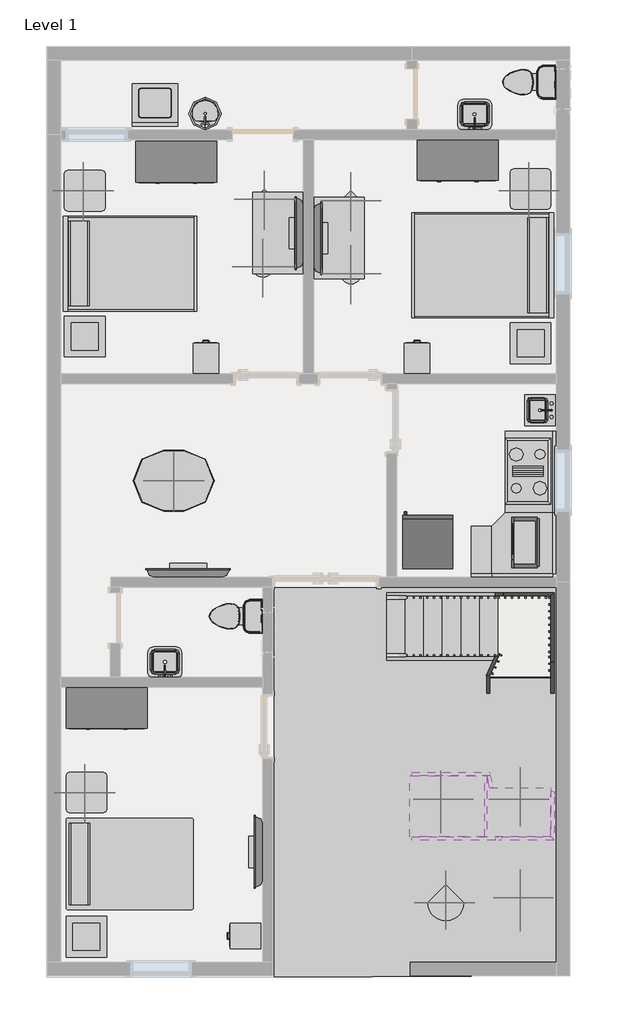
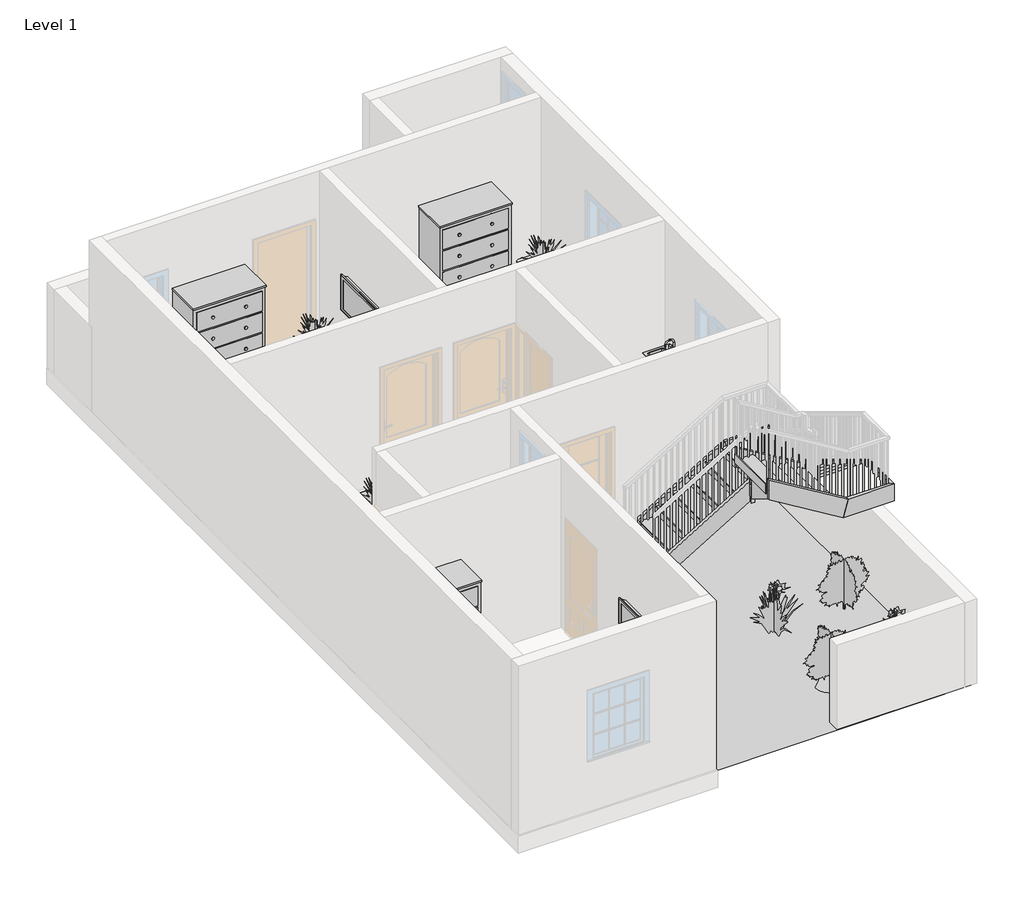
# One storey, part 4 of 4: 23 furniture elements, 12 geographic elements, 12 members, 9 flow terminals, 5 proxies, 3 stair flights, 2 slabs.
"""IFC4 building model written with IfcOpenShell, lengths in millimetres."""

from ifc_helpers import new_model, si_unit, frame, origin, place, context, project, spatial, polyline, outline, extrude, faceted_brep, triangles, transform, mapped, element, save
from components import proxy_bb1e6e30, proxy_8a8d5ab2, proxy_a13a33b2, proxy_718fa39f, flow_terminal_accce45a, flow_terminal_871c2e40, flow_terminal_d49f872f, flow_terminal_62a433f7, toilet_domestic_3d_toilet_domestic_3d_f7549cf7, toilet_domestic_3d_toilet_domestic_3d_183bbd19, furniture_096e7f55, furniture_35c09872, furniture_0253826f, furniture_bb55ed6b, furniture_9fa109b2, furniture_7a3aaa4f, furniture_fdf74506, furniture_b5c51a22, furniture_be1c6672, furniture_31d08a24, furniture_3f969c1c, furniture_25b31cd6, rpc_plant_tropical_55f6ff97, rpc_plant_tropical_agave_1_5_93a2a214, rpc_plant_tropical_jungle_flame_3_9c4808c2, non_monolithic_landing_39c3fcf1, non_monolithic_landing_1f105fa5, stair_flight_290ad292, stair_flight_6c6ed0d7, stair_flight_c4ab4097

model = new_model("IFC4")

# Units and contexts
model_context = context("Model", 3, world=origin())
ifc_project = project(units=[si_unit("LENGTHUNIT", "METRE", prefix="MILLI")], contexts=[model_context])

# Site, building, storey
site = spatial("IfcSite", under=ifc_project)
building = spatial("IfcBuilding", under=site)
storey = spatial("IfcBuildingStorey", under=building, Name="Level 1", Elevation=0.0)

# Proxies
placement = place(None, origin())
element("IfcBuildingElementProxy", 1, Name="Building Element Proxy", at=placement, inside=storey, context=model_context, shape_type="Tessellation", body=[
    triangles([(-10921.0113007, 5381.5366333, 0.0), (-6488.7120758, 5381.5366333, 0.0), (-6488.7120758, -435.0631608, 0.0), (-10921.0113007, -460.4631366, 0.0)], [[1, 4, 3], [3, 2, 1]], closed=False),
])
proxy_shape = proxy_bb1e6e30(model_context)
element("IfcBuildingElementProxy", 2, Name="Cook Top-4 Unit : 36\" x 20\"", ObjectType="Cook Top-4 Unit : 36\" x 20\"", at=placement, inside=storey, context=model_context, shape_type="MappedRepresentation", body=[
    mapped(proxy_shape, transform((-7111.0118598, 7121.4368529, 0.0), x_axis=(0.0, -1.0000000000000004, 0.0), y_axis=(1.0000000000000004, 0.0, 0.0), z_axis=(0.0, 0.0, 1.0))),
])
proxy_2_shape = proxy_8a8d5ab2(model_context)
element("IfcBuildingElementProxy", 3, Name="Microwave : 30\" x 16\" x 18\"", ObjectType="Microwave : 30\" x 16\" x 18\"", at=placement, inside=storey, context=model_context, shape_type="MappedRepresentation", body=[
    mapped(proxy_2_shape, transform((-6796.031354, 6554.9297302, 0.0), x_axis=(0.0, -1.0000000000000004, 0.0), y_axis=(1.0000000000000004, 0.0, 0.0), z_axis=(0.0, 0.0, 1.0))),
])
proxy_3_shape = proxy_a13a33b2(model_context)
element("IfcBuildingElementProxy", 4, Name="Refrigerator : 30\" x 32\" RH", ObjectType="Refrigerator : 30\" x 32\" RH", at=placement, inside=storey, context=model_context, shape_type="MappedRepresentation", body=[
    mapped(proxy_3_shape, transform((-8614.7628883, 6046.6993529, 0.0), x_axis=(-1.0000000000000002, 0.0, 0.0), y_axis=(0.0, -1.0000000000000002, 0.0), z_axis=(0.0, 0.0, 1.0))),
])
proxy_4_shape = proxy_718fa39f(model_context)
element("IfcBuildingElementProxy", 5, Name="Washer : 27\" x 25\" x 35\"", ObjectType="Washer : 27\" x 25\" x 35\"", at=placement, inside=storey, context=model_context, shape_type="MappedRepresentation", body=[
    mapped(proxy_4_shape, transform((-12278.5943913, 12886.9864177, 0.0), x_axis=(-1.0000000000000004, 0.0, 0.0), y_axis=(0.0, -1.0000000000000004, 0.0), z_axis=(0.0, 0.0, 1.0))),
])

# Flow terminals
flow_terminal_shape = flow_terminal_accce45a(model_context)
element("IfcFlowTerminal", 6, ObjectType="Floor Drain - Round : 5\" Strainer - 2\" Drain", at=placement, inside=storey, context=model_context, shape_type="MappedRepresentation", body=[
    mapped(flow_terminal_shape, transform((-12178.3118598, 13077.7368529, 0.0), x_axis=(1.0, 0.0, 0.0), y_axis=(0.0, 1.0, 0.0), z_axis=(0.0, 0.0, 1.0))),
])
element("IfcFlowTerminal", 7, ObjectType="Floor Drain - Round : 5\" Strainer - 2\" Drain", at=placement, inside=storey, context=model_context, shape_type="MappedRepresentation", body=[
    mapped(flow_terminal_shape, transform((-7682.5118598, 13153.9368529, 0.0), x_axis=(1.0, 0.0, 0.0), y_axis=(0.0, 1.0, 0.0), z_axis=(0.0, 0.0, 1.0))),
])
element("IfcFlowTerminal", 8, ObjectType="Floor Drain - Round : 5\" Strainer - 2\" Drain", at=placement, inside=storey, context=model_context, shape_type="MappedRepresentation", body=[
    mapped(flow_terminal_shape, transform((-11441.7118598, 4238.5368529, 0.0), x_axis=(1.0, 0.0, 0.0), y_axis=(0.0, 1.0, 0.0), z_axis=(0.0, 0.0, 1.0))),
])
flow_terminal_2_shape = flow_terminal_871c2e40(model_context)
element("IfcFlowTerminal", 9, ObjectType="Sink Kitchen-Island : 18\" x 18\"", at=placement, inside=storey, context=model_context, shape_type="MappedRepresentation", body=[
    mapped(flow_terminal_2_shape, transform((-6935.5572609, 8051.5260934, 0.0), x_axis=(0.0, -1.0, 0.0), y_axis=(1.0, 0.0, 0.0), z_axis=(0.0, 0.0, 1.0))),
])
flow_terminal_3_shape = flow_terminal_d49f872f(model_context)
element("IfcFlowTerminal", 10, ObjectType="Sink Vanity-Round : 19\" x 19\"", at=placement, inside=storey, context=model_context, shape_type="MappedRepresentation", body=[
    mapped(flow_terminal_3_shape, transform((-11853.0601192, 12566.2547206, 0.0), x_axis=(-1.0000000000000004, 0.0, 0.0), y_axis=(0.0, -1.0000000000000004, 0.0), z_axis=(0.0, 0.0, 1.0))),
])
flow_terminal_4_shape = flow_terminal_62a433f7(model_context)
element("IfcFlowTerminal", 11, ObjectType="Sink Vanity-Square : 20\" x 18\"", at=placement, inside=storey, context=model_context, shape_type="MappedRepresentation", body=[
    mapped(flow_terminal_4_shape, transform((-7895.4226192, 12419.682254, 0.0), x_axis=(-1.0000000000000002, 0.0, 0.0), y_axis=(0.0, -1.0000000000000002, 0.0), z_axis=(0.0, 0.0, 1.0))),
])
element("IfcFlowTerminal", 12, ObjectType="Sink Vanity-Square : 20\" x 18\"", at=placement, inside=storey, context=model_context, shape_type="MappedRepresentation", body=[
    mapped(flow_terminal_4_shape, transform((-12536.3431487, 4215.482254, 0.0), x_axis=(-1.0, 0.0, 0.0), y_axis=(0.0, -1.0, 0.0), z_axis=(0.0, 0.0, 1.0))),
])
toilet_domestic_3d_toilet_domestic_3d_shape = toilet_domestic_3d_toilet_domestic_3d_f7549cf7(model_context)
toilet_domestic_3d_toilet_domestic_3d_2_shape = toilet_domestic_3d_toilet_domestic_3d_183bbd19(model_context)
element("IfcFlowTerminal", 13, ObjectType="Toilet-Domestic-3D : Toilet-Domestic-3D", at=placement, inside=storey, context=model_context, shape_type="MappedRepresentation", body=[
    mapped(toilet_domestic_3d_toilet_domestic_3d_shape, transform((-7186.6078871, 12950.7368529, 0.0), x_axis=(0.0, -1.0000000000000004, 0.0), y_axis=(1.0000000000000004, 0.0, 0.0), z_axis=(0.0, 0.0, 1.0))),
    mapped(toilet_domestic_3d_toilet_domestic_3d_2_shape, transform((-7186.6078871, 12950.7368529, 0.0), x_axis=(0.0, -1.0000000000000004, 0.0), y_axis=(1.0000000000000004, 0.0, 0.0), z_axis=(0.0, 0.0, 1.0))),
])
element("IfcFlowTerminal", 14, ObjectType="Toilet-Domestic-3D : Toilet-Domestic-3D", at=placement, inside=storey, context=model_context, shape_type="MappedRepresentation", body=[
    mapped(toilet_domestic_3d_toilet_domestic_3d_shape, transform((-11580.8078871, 4949.7368529, 0.0), x_axis=(0.0, -1.0000000000000004, 0.0), y_axis=(1.0000000000000004, 0.0, 0.0), z_axis=(0.0, 0.0, 1.0))),
    mapped(toilet_domestic_3d_toilet_domestic_3d_2_shape, transform((-11580.8078871, 4949.7368529, 0.0), x_axis=(0.0, -1.0000000000000004, 0.0), y_axis=(1.0000000000000004, 0.0, 0.0), z_axis=(0.0, 0.0, 1.0))),
])

# Furniture
furniture_shape = furniture_096e7f55(model_context)
element("IfcFurniture", 15, ObjectType="Bed-Shaker : Double 56\" x 78\"", at=placement, inside=storey, context=model_context, shape_type="MappedRepresentation", body=[
    mapped(furniture_shape, transform((-14057.9118598, 10251.9868529, 0.0), x_axis=(0.0, 1.0000000000000002, 0.0), y_axis=(-1.0000000000000002, 0.0, 0.0), z_axis=(0.0, 0.0, 1.0))),
])
furniture_2_shape = furniture_35c09872(model_context)
element("IfcFurniture", 16, ObjectType="Bed-Shaker : Queen 62\" x 83\"", at=placement, inside=storey, context=model_context, shape_type="MappedRepresentation", body=[
    mapped(furniture_2_shape, transform((-6742.7118598, 10188.4868529, 0.0), x_axis=(0.0, -1.0, 0.0), y_axis=(1.0, 0.0, 0.0), z_axis=(0.0, 0.0, 1.0))),
])
furniture_3_shape = furniture_0253826f(model_context)
element("IfcFurniture", 17, ObjectType="Bed-Standard : Double 54\" x 75\"", at=placement, inside=storey, context=model_context, shape_type="MappedRepresentation", body=[
    mapped(furniture_3_shape, transform((-13125.6069417, 969.8483283, 0.0), x_axis=(0.0, 1.0, 0.0), y_axis=(-1.0, 0.0, 0.0), z_axis=(0.0, 0.0, 1.0))),
])
furniture_4_shape = furniture_bb55ed6b(model_context)
element("IfcFurniture", 18, ObjectType="Cabinet-File 2 Drawer : 15\" x 18\"", at=placement, inside=storey, context=model_context, shape_type="MappedRepresentation", body=[
    mapped(furniture_4_shape, transform((-12064.9083068, 8668.4025527, 0.0), x_axis=(-1.0000000000000009, 0.0, 0.0), y_axis=(0.0, -1.0000000000000009, 0.0), z_axis=(0.0, 0.0, 1.0))),
])
element("IfcFurniture", 19, ObjectType="Cabinet-File 2 Drawer : 15\" x 18\"", at=placement, inside=storey, context=model_context, shape_type="MappedRepresentation", body=[
    mapped(furniture_4_shape, transform((-8902.6083068, 8668.4025527, 0.0), x_axis=(-1.0, 0.0, 0.0), y_axis=(0.0, -1.0, 0.0), z_axis=(0.0, 0.0, 1.0))),
])
element("IfcFurniture", 20, ObjectType="Cabinet-File 2 Drawer : 15\" x 18\"", at=placement, inside=storey, context=model_context, shape_type="MappedRepresentation", body=[
    mapped(furniture_4_shape, transform((-11204.3275597, 33.9404058, 0.0), x_axis=(0.0, -0.9999999999999997, 0.0), y_axis=(0.9999999999999997, 0.0, 0.0), z_axis=(0.0, 0.0, 1.0))),
])
furniture_5_shape = furniture_9fa109b2(model_context)
element("IfcFurniture", 21, ObjectType="Dresser : 48\" x 72\" x 24\"", at=placement, inside=storey, context=model_context, shape_type="MappedRepresentation", body=[
    mapped(furniture_5_shape, transform((-12112.3185999, 12120.099807, 0.0), x_axis=(1.0000000000000007, 0.0, 0.0), y_axis=(0.0, 1.0000000000000007, 0.0), z_axis=(0.0, 0.0, 1.0))),
])
element("IfcFurniture", 22, ObjectType="Dresser : 48\" x 72\" x 24\"", at=placement, inside=storey, context=model_context, shape_type="MappedRepresentation", body=[
    mapped(furniture_5_shape, transform((-7895.9185999, 12145.499807, 0.0), x_axis=(1.0, 0.0, 0.0), y_axis=(0.0, 1.0, 0.0), z_axis=(0.0, 0.0, 1.0))),
])
element("IfcFurniture", 23, ObjectType="Dresser : 48\" x 72\" x 24\"", at=placement, inside=storey, context=model_context, shape_type="MappedRepresentation", body=[
    mapped(furniture_5_shape, transform((-13153.7185999, 3941.299807, 0.0), x_axis=(1.0, 0.0, 0.0), y_axis=(0.0, 1.0, 0.0), z_axis=(0.0, 0.0, 1.0))),
])
furniture_6_shape = furniture_7a3aaa4f(model_context)
element("IfcFurniture", 24, ObjectType="TV - Flat Screen : 42\"", at=placement, inside=storey, context=model_context, shape_type="MappedRepresentation", body=[
    mapped(furniture_6_shape, transform((-10535.0504834, 10686.1923387, 1041.4), x_axis=(0.0, -1.0000000000000004, 0.0), y_axis=(1.0000000000000004, 0.0, 0.0), z_axis=(0.0, 0.0, 1.0))),
])
element("IfcFurniture", 25, ObjectType="TV - Flat Screen : 42\"", at=placement, inside=storey, context=model_context, shape_type="MappedRepresentation", body=[
    mapped(furniture_6_shape, transform((-10265.5732361, 10617.881367, 1041.4), x_axis=(0.0, 1.0000000000000002, 0.0), y_axis=(-1.0000000000000002, 0.0, 0.0), z_axis=(0.0, 0.0, 1.0))),
])
element("IfcFurniture", 26, ObjectType="TV - Flat Screen : 42\"", at=placement, inside=storey, context=model_context, shape_type="MappedRepresentation", body=[
    mapped(furniture_6_shape, transform((-11144.6504834, 1415.1923387, 1041.4), x_axis=(0.0, -1.0000000000000004, 0.0), y_axis=(1.0000000000000004, 0.0, 0.0), z_axis=(0.0, 0.0, 1.0))),
])
furniture_7_shape = furniture_fdf74506(model_context)
element("IfcFurniture", 27, ObjectType="TV - Flat Screen : 50\"", at=placement, inside=storey, context=model_context, shape_type="MappedRepresentation", body=[
    mapped(furniture_7_shape, transform((-12207.6563739, 5592.4754765, 1041.4), x_axis=(-1.0000000000000004, 0.0, 0.0), y_axis=(0.0, -1.0000000000000004, 0.0), z_axis=(0.0, 0.0, 1.0))),
])
furniture_8_shape = furniture_b5c51a22(model_context)
element("IfcFurniture", 28, ObjectType="Table-Coffee : 24\" x 24\" x 24\"", at=placement, inside=storey, context=model_context, shape_type="MappedRepresentation", body=[
    mapped(furniture_8_shape, transform((-13771.3776265, 9045.5257751, 0.0), x_axis=(1.0, 0.0, 0.0), y_axis=(0.0, 1.0, 0.0), z_axis=(0.0, 0.0, 1.0))),
])
element("IfcFurniture", 29, ObjectType="Table-Coffee : 24\" x 24\" x 24\"", at=placement, inside=storey, context=model_context, shape_type="MappedRepresentation", body=[
    mapped(furniture_8_shape, transform((-7091.1776265, 8943.9257751, 0.0), x_axis=(1.0, 0.0, 0.0), y_axis=(0.0, 1.0, 0.0), z_axis=(0.0, 0.0, 1.0))),
])
element("IfcFurniture", 30, ObjectType="Table-Coffee : 24\" x 24\" x 24\"", at=placement, inside=storey, context=model_context, shape_type="MappedRepresentation", body=[
    mapped(furniture_8_shape, transform((-13745.9776265, 53.9257751, 0.0), x_axis=(1.0, 0.0, 0.0), y_axis=(0.0, 1.0, 0.0), z_axis=(0.0, 0.0, 1.0))),
])
furniture_9_shape = furniture_be1c6672(model_context)
element("IfcFurniture", 31, ObjectType="Table-Dining Oval : 36\" x 48\"", at=placement, inside=storey, context=model_context, shape_type="MappedRepresentation", body=[
    mapped(furniture_9_shape, transform((-12821.4315319, 6623.6384922, 0.0), x_axis=(-1.0000000000000004, 0.0, 0.0), y_axis=(0.0, -1.0000000000000004, 0.0), z_axis=(0.0, 0.0, 1.0))),
])
furniture_10_shape = furniture_31d08a24(model_context)
element("IfcFurniture", 32, ObjectType="Table-End : 24\" x 24\"", at=placement, inside=storey, context=model_context, shape_type="MappedRepresentation", body=[
    mapped(furniture_10_shape, transform((-14061.6454901, 11172.7368529, 0.0), x_axis=(1.0, 0.0, 0.0), y_axis=(0.0, 1.0, 0.0), z_axis=(0.0, 0.0, 1.0))),
])
element("IfcFurniture", 33, ObjectType="Table-End : 24\" x 24\"", at=placement, inside=storey, context=model_context, shape_type="MappedRepresentation", body=[
    mapped(furniture_10_shape, transform((-7381.4454901, 11198.1368529, 0.0), x_axis=(1.0, 0.0, 0.0), y_axis=(0.0, 1.0, 0.0), z_axis=(0.0, 0.0, 1.0))),
])
element("IfcFurniture", 34, ObjectType="Table-End : 24\" x 24\"", at=placement, inside=storey, context=model_context, shape_type="MappedRepresentation", body=[
    mapped(furniture_10_shape, transform((-14036.2454901, 2155.7368529, 0.0), x_axis=(1.0, 0.0, 0.0), y_axis=(0.0, 1.0, 0.0), z_axis=(0.0, 0.0, 1.0))),
])
furniture_11_shape = furniture_3f969c1c(model_context)
element("IfcFurniture", 35, ObjectType="Table-Rectangular : 72\" x 30\"", at=placement, inside=storey, context=model_context, shape_type="MappedRepresentation", body=[
    mapped(furniture_11_shape, transform((-10857.5118598, 10690.1368529, 0.0), x_axis=(0.0, 1.0000000000000002, 0.0), y_axis=(-1.0000000000000002, 0.0, 0.0), z_axis=(0.0, 0.0, 1.0))),
])
element("IfcFurniture", 36, ObjectType="Table-Rectangular : 72\" x 30\"", at=placement, inside=storey, context=model_context, shape_type="MappedRepresentation", body=[
    mapped(furniture_11_shape, transform((-9943.1118598, 10613.9368529, 0.0), x_axis=(0.0, 1.0000000000000002, 0.0), y_axis=(-1.0000000000000002, 0.0, 0.0), z_axis=(0.0, 0.0, 1.0))),
])
furniture_12_shape = furniture_25b31cd6(model_context)
element("IfcFurniture", 37, ObjectType="Work Station Cubicle : 96\" x 96\"", at=placement, inside=storey, context=model_context, shape_type="MappedRepresentation", body=[
    mapped(furniture_12_shape, transform((-6823.643612, 5038.9138452, 0.0), x_axis=(-1.0000000000000004, 0.0, 0.0), y_axis=(0.0, -1.0000000000000004, 0.0), z_axis=(0.0, 0.0, 1.0))),
])

# Geographic elements
rpc_plant_tropical_shape = rpc_plant_tropical_55f6ff97(model_context)
element("IfcGeographicElement", 38, ObjectType="RPC Plant - Tropical", at=placement, inside=storey, context=model_context, shape_type="MappedRepresentation", body=[
    mapped(rpc_plant_tropical_shape, transform((-8419.1118598, 2206.5368529, 0.0), x_axis=(1.0, 0.0, 0.0), y_axis=(0.0, 1.0, 0.0), z_axis=(0.0, 0.0, 1.0))),
])
element("IfcGeographicElement", 39, ObjectType="RPC Plant - Tropical", at=placement, inside=storey, context=model_context, shape_type="MappedRepresentation", body=[
    mapped(rpc_plant_tropical_shape, transform((-7225.3118598, 733.3368529, 0.0), x_axis=(1.0, 0.0, 0.0), y_axis=(0.0, 1.0, 0.0), z_axis=(0.0, 0.0, 1.0))),
])
rpc_plant_tropical_agave_1_5_shape = rpc_plant_tropical_agave_1_5_93a2a214(model_context)
element("IfcGeographicElement", 40, ObjectType="RPC Plant - Tropical : Agave - 1.5'", at=placement, inside=storey, context=model_context, shape_type="MappedRepresentation", body=[
    mapped(rpc_plant_tropical_agave_1_5_shape, transform((-13778.5118598, 11325.1368529, 609.6), x_axis=(1.0, 0.0, 0.0), y_axis=(0.0, 1.0, 0.0), z_axis=(0.0, 0.0, 1.0))),
])
element("IfcGeographicElement", 41, ObjectType="RPC Plant - Tropical : Agave - 1.5'", at=placement, inside=storey, context=model_context, shape_type="MappedRepresentation", body=[
    mapped(rpc_plant_tropical_agave_1_5_shape, transform((-11060.7118598, 11198.1368529, 660.4), x_axis=(1.0, 0.0, 0.0), y_axis=(0.0, 1.0, 0.0), z_axis=(0.0, 0.0, 1.0))),
])
element("IfcGeographicElement", 42, ObjectType="RPC Plant - Tropical : Agave - 1.5'", at=placement, inside=storey, context=model_context, shape_type="MappedRepresentation", body=[
    mapped(rpc_plant_tropical_agave_1_5_shape, transform((-11086.1118598, 10182.1368529, 660.4), x_axis=(1.0, 0.0, 0.0), y_axis=(0.0, 1.0, 0.0), z_axis=(0.0, 0.0, 1.0))),
])
element("IfcGeographicElement", 43, ObjectType="RPC Plant - Tropical : Agave - 1.5'", at=placement, inside=storey, context=model_context, shape_type="MappedRepresentation", body=[
    mapped(rpc_plant_tropical_agave_1_5_shape, transform((-7098.3118598, 11325.1368529, 609.6), x_axis=(1.0, 0.0, 0.0), y_axis=(0.0, 1.0, 0.0), z_axis=(0.0, 0.0, 1.0))),
])
element("IfcGeographicElement", 44, ObjectType="RPC Plant - Tropical : Agave - 1.5'", at=placement, inside=storey, context=model_context, shape_type="MappedRepresentation", body=[
    mapped(rpc_plant_tropical_agave_1_5_shape, transform((-9765.3118598, 11172.7368529, 660.4), x_axis=(1.0, 0.0, 0.0), y_axis=(0.0, 1.0, 0.0), z_axis=(0.0, 0.0, 1.0))),
])
element("IfcGeographicElement", 45, ObjectType="RPC Plant - Tropical : Agave - 1.5'", at=placement, inside=storey, context=model_context, shape_type="MappedRepresentation", body=[
    mapped(rpc_plant_tropical_agave_1_5_shape, transform((-9765.3118598, 10080.5368529, 660.4), x_axis=(1.0, 0.0, 0.0), y_axis=(0.0, 1.0, 0.0), z_axis=(0.0, 0.0, 1.0))),
])
element("IfcGeographicElement", 46, ObjectType="RPC Plant - Tropical : Agave - 1.5'", at=placement, inside=storey, context=model_context, shape_type="MappedRepresentation", body=[
    mapped(rpc_plant_tropical_agave_1_5_shape, transform((-12419.6118598, 6981.7368529, 736.6), x_axis=(1.0, 0.0, 0.0), y_axis=(0.0, 1.0, 0.0), z_axis=(0.0, 0.0, 1.0))),
])
element("IfcGeographicElement", 47, ObjectType="RPC Plant - Tropical : Agave - 1.5'", at=placement, inside=storey, context=model_context, shape_type="MappedRepresentation", body=[
    mapped(rpc_plant_tropical_agave_1_5_shape, transform((-13753.1118598, 2308.1368529, 609.6), x_axis=(1.0, 0.0, 0.0), y_axis=(0.0, 1.0, 0.0), z_axis=(0.0, 0.0, 1.0))),
])
rpc_plant_tropical_jungle_flame_3_shape = rpc_plant_tropical_jungle_flame_3_9c4808c2(model_context)
element("IfcGeographicElement", 48, ObjectType="RPC Plant - Tropical : Jungle Flame - 3'", at=placement, inside=storey, context=model_context, shape_type="MappedRepresentation", body=[
    mapped(rpc_plant_tropical_jungle_flame_3_shape, transform((-7225.3118598, 2206.5368529, 0.0), x_axis=(1.0, 0.0, 0.0), y_axis=(0.0, 1.0, 0.0), z_axis=(0.0, 0.0, 1.0))),
])
element("IfcGeographicElement", 49, ObjectType="RPC Plant - Tropical : Jungle Flame - 3'", at=placement, inside=storey, context=model_context, shape_type="MappedRepresentation", body=[
    mapped(rpc_plant_tropical_jungle_flame_3_shape, transform((-8342.9118598, 657.1368529, 0.0), x_axis=(1.0, 0.0, 0.0), y_axis=(0.0, 1.0, 0.0), z_axis=(0.0, 0.0, 1.0))),
])

# Members
element("IfcMember", 50, ObjectType="Stringer - 2\" Width", at=placement, inside=storey, context=model_context, shape_type="SweptSolid", body=[
    extrude(outline(polyline([(212.114512, -9231.9118598), (0.0, -9231.9118598), (0.0, -8993.826348), (956.7333333, -7415.216348), (1261.5333333, -7500.3708045), (212.114512, -9231.9118598)])), frame((0.0, 5254.5368529, 0.0), z_axis=(0.0, 1.0, 0.0), x_axis=(0.0, 0.0, 1.0)), (0.0, 0.0, 1.0), 50.8),
])
element("IfcMember", 51, ObjectType="Stringer - 2\" Width", at=placement, inside=storey, context=model_context, shape_type="Brep", body=[
    faceted_brep([(-9231.9118598, 4289.3368529, 0.0), (-9231.9118598, 4340.1368529, 0.0), (-8993.826348, 4340.1368529, 0.0), (-8993.826348, 4289.3368529, 0.0), (-9231.9118598, 4289.3368529, 212.114512), (-9231.9118598, 4340.1368529, 212.114512), (-7634.4044721, 4289.3368529, 1180.3008075), (-7611.313563, 4340.1368529, 1194.2952979), (-7611.313563, 4340.1368529, 837.8865364), (-7634.4044721, 4289.3368529, 823.892046)], [[[0, 1, 2, 3]], [[4, 5, 1, 0]], [[5, 4, 6, 7]], [[1, 5, 7, 8, 2]], [[4, 0, 3, 9, 6]], [[2, 8, 9, 3]], [[6, 9, 8, 7]]]),
])
element("IfcMember", 52, ObjectType="Stringer - 2\" Width", at=placement, inside=storey, context=model_context, shape_type="SweptSolid", body=[
    extrude(outline(polyline([(4284.9957976, 1261.5333333), (4199.8413411, 956.7333333), (2244.0413411, 2142.0666667), (2329.1957976, 2446.8666667), (4284.9957976, 1261.5333333)])), frame((-6768.1118598, 0.0, 0.0), z_axis=(1.0, 0.0, 0.0), x_axis=(0.0, 1.0, 0.0)), (0.0, 0.0, 1.0), 50.8),
])
element("IfcMember", 53, ObjectType="Stringer - 2\" Width", at=placement, inside=storey, context=model_context, shape_type="SweptSolid", body=[
    extrude(outline(polyline([(4060.7368529, 1397.4478453), (4060.7368529, 1041.0390838), (2384.3368529, 2057.0390838), (2384.3368529, 2413.4478453), (4060.7368529, 1397.4478453)])), frame((-7733.3118598, 0.0, 0.0), z_axis=(1.0, 0.0, 0.0), x_axis=(0.0, 1.0, 0.0)), (0.0, 0.0, 1.0), 50.8),
])
element("IfcMember", 54, ObjectType="Stringer - 2\" Width", at=placement, inside=storey, context=model_context, shape_type="Brep", body=[
    faceted_brep([(-6768.1118598, 4284.9957976, 1261.5333333), (-6717.3118598, 4284.9957976, 1261.5333333), (-6717.3118598, 5305.3368529, 1261.5333333), (-6768.1118598, 5254.5368529, 1261.5333333), (-6768.1118598, 4199.8413411, 956.7333333), (-6768.1118598, 5254.5368529, 956.7333333), (-6717.3118598, 4199.8413411, 956.7333333), (-6717.3118598, 5305.3368529, 956.7333333)], [[[0, 1, 2, 3]], [[4, 0, 3, 5]], [[6, 4, 5, 7]], [[1, 6, 7, 2]], [[1, 0, 4, 6]], [[2, 7, 5, 3]]]),
])
element("IfcMember", 55, ObjectType="Stringer - 2\" Width", at=placement, inside=storey, context=model_context, shape_type="Brep", body=[
    faceted_brep([(-6768.1118598, 5254.5368529, 1261.5333333), (-6717.3118598, 5305.3368529, 1261.5333333), (-7500.3708045, 5305.3368529, 1261.5333333), (-7500.3708045, 5254.5368529, 1261.5333333), (-6768.1118598, 5254.5368529, 956.7333333), (-7415.216348, 5254.5368529, 956.7333333), (-6717.3118598, 5305.3368529, 956.7333333), (-7415.216348, 5305.3368529, 956.7333333)], [[[0, 1, 2, 3]], [[4, 0, 3, 5]], [[6, 4, 5, 7]], [[1, 6, 7, 2]], [[1, 0, 4, 6]], [[2, 7, 5, 3]]]),
])
element("IfcMember", 56, ObjectType="Stringer - 2\" Width", at=placement, inside=storey, context=model_context, shape_type="SweptSolid", body=[
    extrude(outline(polyline([(-7611.313563, 4340.1368529), (-7555.5118598, 4340.1368529), (-7682.5118598, 4060.7368529), (-7738.313563, 4060.7368529), (-7611.313563, 4340.1368529)])), frame((0.0, 0.0, 956.7333333), z_axis=(0.0, 0.0, 1.0), x_axis=(1.0, 0.0, 0.0)), (0.0, 0.0, 1.0), 304.8),
])
element("IfcMember", 57, ObjectType="Stringer - 2\" Width", at=placement, inside=storey, context=model_context, shape_type="SweptSolid", body=[
    extrude(outline(polyline([(2142.0666667, -7594.2073716), (2446.8666667, -7509.052915), (3260.114512, -8850.9118598), (2903.7057504, -8850.9118598), (2142.0666667, -7594.2073716)])), frame((0.0, 1596.9368529, 0.0), z_axis=(0.0, 1.0, 0.0), x_axis=(0.0, 0.0, 1.0)), (0.0, 0.0, 1.0), 50.8),
])
element("IfcMember", 58, ObjectType="Stringer - 2\" Width", at=placement, inside=storey, context=model_context, shape_type="Brep", body=[
    faceted_brep([(-8850.9118598, 2612.9368529, 3260.114512), (-8850.9118598, 2612.9368529, 2903.7057504), (-8850.9118598, 2562.1368529, 2903.7057504), (-8850.9118598, 2562.1368529, 3260.114512), (-7680.4790623, 2562.1368529, 2550.7613014), (-7694.993348, 2612.9368529, 2559.5578382), (-7680.4790623, 2562.1368529, 2194.3525398), (-7694.993348, 2612.9368529, 2203.1490766)], [[[0, 1, 2, 3]], [[4, 5, 0, 3]], [[6, 4, 3, 2]], [[7, 6, 2, 1]], [[5, 7, 1, 0]], [[5, 4, 6, 7]]]),
])
element("IfcMember", 59, ObjectType="Stringer - 2\" Width", at=placement, inside=storey, context=model_context, shape_type="Brep", body=[
    faceted_brep([(-7509.052915, 1647.7368529, 2446.8666667), (-7509.052915, 1596.9368529, 2446.8666667), (-6717.3118598, 1596.9368529, 2446.8666667), (-6768.1118598, 1647.7368529, 2446.8666667), (-7594.2073716, 1647.7368529, 2142.0666667), (-6768.1118598, 1647.7368529, 2142.0666667), (-7594.2073716, 1596.9368529, 2142.0666667), (-6717.3118598, 1596.9368529, 2142.0666667)], [[[0, 1, 2, 3]], [[4, 0, 3, 5]], [[6, 4, 5, 7]], [[1, 6, 7, 2]], [[1, 0, 4, 6]], [[2, 7, 5, 3]]]),
])
element("IfcMember", 60, ObjectType="Stringer - 2\" Width", at=placement, inside=storey, context=model_context, shape_type="Brep", body=[
    faceted_brep([(-6768.1118598, 1647.7368529, 2446.8666667), (-6717.3118598, 1596.9368529, 2446.8666667), (-6717.3118598, 2329.1957976, 2446.8666667), (-6768.1118598, 2329.1957976, 2446.8666667), (-6768.1118598, 1647.7368529, 2142.0666667), (-6768.1118598, 2244.0413411, 2142.0666667), (-6717.3118598, 1596.9368529, 2142.0666667), (-6717.3118598, 2244.0413411, 2142.0666667)], [[[0, 1, 2, 3]], [[4, 0, 3, 5]], [[6, 4, 5, 7]], [[1, 6, 7, 2]], [[1, 0, 4, 6]], [[2, 7, 5, 3]]]),
])
element("IfcMember", 61, ObjectType="Stringer - 2\" Width", at=placement, inside=storey, context=model_context, shape_type="SweptSolid", body=[
    extrude(outline(polyline([(-7629.6790623, 2384.3368529), (-7682.5118598, 2384.3368529), (-7733.3118598, 2562.1368529), (-7680.4790623, 2562.1368529), (-7629.6790623, 2384.3368529)])), frame((0.0, 0.0, 2142.0666667), z_axis=(0.0, 0.0, 1.0), x_axis=(1.0, 0.0, 0.0)), (0.0, 0.0, 1.0), 304.8),
])

# Slabs
non_monolithic_landing_shape = non_monolithic_landing_39c3fcf1(model_context)
element("IfcSlab", 62, ObjectType="Non-Monolithic Landing", at=placement, inside=storey, context=model_context, shape_type="MappedRepresentation", body=[
    mapped(non_monolithic_landing_shape, transform((0.0, 0.0, 0.0), x_axis=(1.0, 0.0, 0.0), y_axis=(0.0, 1.0, 0.0), z_axis=(0.0, 0.0, 1.0))),
])
non_monolithic_landing_2_shape = non_monolithic_landing_1f105fa5(model_context)
element("IfcSlab", 63, ObjectType="Non-Monolithic Landing", at=placement, inside=storey, context=model_context, shape_type="MappedRepresentation", body=[
    mapped(non_monolithic_landing_2_shape, transform((0.0, 0.0, 0.0), x_axis=(1.0, 0.0, 0.0), y_axis=(0.0, 1.0, 0.0), z_axis=(0.0, 0.0, 1.0))),
])

# Stair flights
stair_flight_shape = stair_flight_290ad292(model_context)
element("IfcStairFlight", 64, ObjectType="2\" Tread 1\" Nosing 1/4\" Riser", at=placement, inside=storey, context=model_context, shape_type="MappedRepresentation", body=[
    mapped(stair_flight_shape, transform((0.0, 0.0, 0.0), x_axis=(1.0, 0.0, 0.0), y_axis=(0.0, 1.0, 0.0), z_axis=(0.0, 0.0, 1.0))),
])
stair_flight_2_shape = stair_flight_6c6ed0d7(model_context)
element("IfcStairFlight", 65, ObjectType="2\" Tread 1\" Nosing 1/4\" Riser", at=placement, inside=storey, context=model_context, shape_type="MappedRepresentation", body=[
    mapped(stair_flight_2_shape, transform((0.0, 0.0, 0.0), x_axis=(1.0, 0.0, 0.0), y_axis=(0.0, 1.0, 0.0), z_axis=(0.0, 0.0, 1.0))),
])
stair_flight_3_shape = stair_flight_c4ab4097(model_context)
element("IfcStairFlight", 66, ObjectType="2\" Tread 1\" Nosing 1/4\" Riser", at=placement, inside=storey, context=model_context, shape_type="MappedRepresentation", body=[
    mapped(stair_flight_3_shape, transform((0.0, 0.0, 0.0), x_axis=(1.0, 0.0, 0.0), y_axis=(0.0, 1.0, 0.0), z_axis=(0.0, 0.0, 1.0))),
])

save(model, "model.ifc")

# Revit data of these elements
# Type "Cook Top-4 Unit : 36\" x 20\""
#   Assembly Code = "E1090400"
#   Depth = 2' - 0"
#   Width = 3' - 0"
#   Burner Material = Steel, Chrome Plated
#   Cooktop Material = Steel, Polished
#   Default Elevation = 0
# Type "Microwave : 30\" x 16\" x 18\""
#   Assembly Code = "E1090400"
#   Depth = 1' - 4"
#   Height = 1' - 6"
#   Width = 2' - 6"
#   Microwave Material = Laminate, Linen, Matte
#   Default Elevation = 0
# Type "Refrigerator : 30\" x 32\" RH"
#   Label = "REF."
#   Assembly Code = "E1090400"
#   Depth = 2' - 7 3/4"
#   Handle = 2' - 3"
#   Height = 5' - 10"
#   Rear Clearance = 0' - 2"
#   Top Door Height = 1' - 8"
#   Width = 2' - 5 3/8"
#   Material = Carpet (1)
#   Default Elevation = 0
# Type "Washer : 27\" x 25\" x 35\""
#   Label = "W"
#   Assembly Code = "E1090400"
#   Depth = 2' - 1"
#   Height = 2' - 11"
#   Width = 2' - 3"
#   Washer Material = Steel, Paint Finish, Ivory, Matte
#   Default Elevation = 0
# Type "Floor Drain - Round : 5\" Strainer - 2\" Drain"
#   WFU = 2
#   Strainer Height = 0' - 3 1/4"
#   Strainer Radius = 0' - 2 1/2"
#   Strainer Diameter = 0' - 5"
#   Radius 6 = 0' - 0 5/8"
#   Radius 5 = 0' - 1 1/4"
#   Radius 4 = 0' - 1 7/8"
#   Radius 2 = 0' - 3.04167"
#   Radius 1 = 0' - 2.02083"
#   Radius 3 = 0' - 2 1/32"
#   Pipe Radius = 1"
#   Pipe Diameter = 2"
#   Height 2 = 0' - 0.725"
#   Height 1 = 0' - 1 13/16"
#   Body Radius = 0' - 4 1/16"
#   Body Height = 0' - 3 5/8"
#   Body Diameter = 0' - 8 1/8"
#   Drain Material = none
#   HWFU = 0
#   Default Elevation = 0
#   CWFU = 0
# Type "Sink Kitchen-Island : 18\" x 18\""
#   Assembly Code = "D2010410"
#   Counter Height = 3' - 0"
#   Depth = 1' - 6"
#   Width = 1' - 6"
#   Faucet Material = Steel, Polished
#   Sink Material = Steel, Polished
#   Default Elevation = 0
# Type "Sink Vanity-Round : 19\" x 19\""
#   Assembly Code = "D2010400"
#   Top Of Counter = 2' - 7"
#   Basin Material = Porcelain, Linen
#   Faucet Material = Steel, Polished
#   Default Elevation = 0
# Type "Sink Vanity-Square : 20\" x 18\""
#   Assembly Code = "D2010400"
#   Counter Height = 2' - 7"
#   Depth = 1' - 6"
#   Width = 1' - 8"
#   Basin Material = Porcelain, Linen
#   Faucet Material = Steel, Polished
#   Default Elevation = 0
# Type "Toilet-Domestic-3D : Toilet-Domestic-3D"
#   Assembly Code = "D2010110"
#   Toilet - Bowl/Basin Material = Porcelain, Linen
#   Toilet - Seat Material = Laminate, Linen, Matte
#   Default Elevation = 0
# Type "Bed-Shaker : Double 56\" x 78\""
#   Assembly Code = "E2020200"
#   Length = 6' - 6"
#   Width = 4' - 8"
#   Frame Material = Birch
#   Mattress Material = Sash
#   Default Elevation = 0
# Type "Bed-Shaker : Queen 62\" x 83\""
#   Assembly Code = "E2020200"
#   Length = 6' - 11"
#   Width = 5' - 2"
#   Frame Material = Birch
#   Mattress Material = Sash
#   Default Elevation = 0
# Type "Bed-Standard : Double 54\" x 75\""
#   Assembly Code = "E2020200"
#   Length = 6' - 3"
#   Width = 4' - 6"
#   Leg Material = Steel, Chrome Plated
#   Mattress Material = Linen, White
#   Default Elevation = 0
# Type "Cabinet-File 2 Drawer : 15\" x 18\""
#   Assembly Code = "E2020200"
#   Depth = 1' - 6"
#   Height = 2' - 5"
#   Width = 1' - 3"
#   Cabinet Material = Steel, Paint Finish, Ivory, Glossy
#   Handle Material = Steel, Chrome Plated
#   Default Elevation = 0
# Type "Dresser : 48\" x 72\" x 24\""
#   Assembly Code = "E2020200"
#   Depth = 2' - 0"
#   Height = 6' - 0"
#   Width = 4' - 0"
#   Dresser Material = Wood - Teak
#   Drawer Material = Wood - Teak
#   Knob Material = Cherry
#   Default Elevation = 0
# Type "TV - Flat Screen : 42\""
#   SinAng = 0' - 0.0193"
#   L = 3' - 0.71517"
#   H = 1' - 8.65418"
#   Thickness = 0' - 4.33071"
#   Diagonal = 3' - 6.12598"
#   CosAng = 0' - 0.03431"
#   Stand [instance default] = yes
#   Default Elevation = 0
# Type "TV - Flat Screen : 50\""
#   SinAng = 0' - 0.0193"
#   L = 3' - 7.57782"
#   H = 2' - 0.51477"
#   Thickness = 0' - 4.33071"
#   Diagonal = 4' - 2"
#   CosAng = 0' - 0.03431"
#   Stand [instance default] = yes
#   Default Elevation = 0
# Type "Table-Coffee : 24\" x 24\" x 24\""
#   Assembly Code = "E2020200"
#   Height = 2' - 0"
#   Length = 2' - 0"
#   Width = 2' - 0"
#   Top Material = none
#   Frame Material = none
#   Default Elevation = 0
# Type "Table-Dining Oval : 36\" x 48\""
#   Assembly Code = "E2020200"
#   Length = 4' - 0"
#   Width = 3' - 0"
#   Base Material = Steel, Chrome Plated
#   Top Material = Glass - Clear, Grey
#   Default Elevation = 0
#   Description = (empty or 0)
# Type "Table-End : 24\" x 24\""
#   Assembly Code = "E2020200"
#   Height = 2' - 0"
#   Length = 2' - 0"
#   Width = 2' - 0"
#   Base Material = Birch
#   Top Material = Laminate, Ivory, Matte
#   Default Elevation = 0
# Type "Table-Rectangular : 72\" x 30\""
#   Assembly Code = "E2020200"
#   Height = 2' - 2"
#   Length = 4' - 0"
#   Width = 2' - 6"
#   Base Material = Birch
#   Top Material = Birch
#   Default Elevation = 0
# Type "Work Station Cubicle : 96\" x 96\""
#   Assembly Code = "E2020"
#   Desktop Height = 2' - 6"
#   Desktop1 Width = 2' - 4"
#   Desktop2 Width = 2' - 4"
#   Panel Height = 2' - 8"
#   Panel1 Length = 4' - 0"
#   Panel2 Length = 1' - 0"
#   Cube Panel Material = Textile - Light Gray
#   Work Top Material = Laminate, Ivory, Matte
#   Default Elevation = 0
# Type "RPC Plant - Tropical"
#   built-in parameter 1005198 = "{2, 15},{39, RPC-16-FWM5-GM7X-C67P-4000-ST1L-LVER-AU},{1, 0},{1, 0},{2, 13},{1, 8},{5, Color},{1, 0},{1, 0},{3, 0.8},{3, 0.8},{3, 0.8},{1, 8},{7, BBoxMin},{1, 0},{1, 0},{1, 0},{1, 0},{1, 0},{1, 8},{7, BBoxMax},{1, 0},{1, 0},{1, 0},{1, 0},{1, 0},{2, 11},{9, RPCTypeId},{1, 0},{1, 0},{39, RPC-16-FWM5-GM7X-C67P-4000-ST1L-LVER-AU},{1, 6},{14, RPCPlantHeight},{1, 0},{1, 0},{1, 3},{2, 11},{7, keyword},{1, 0},{1, 0},{35, :RPCs:Shrubs [General]:Geometry:RPC},{2, 11},{8, category},{1, 0},{1, 0},{16, Shrubs [General]},{2, 11},{12, LocalizedUID},{1, 0},{1, 0},{10, Crane Lily},{2, 14},{6, Height},{1, 0},{1, 0},{1, 3},{1, 2},{16, Cast Reflections},{1, 0},{1, 0},{1, 0},{1, 2},{12, Cast Shadows},{1, 0},{1, 0},{1, 1},{1, 2},{9, Lock View},{1, 0},{1, 0},{1, 0},{1, 4},{5, ViewC},{1, 0},{1, 0},{1, 0},{21, assetlibrary_base.fbx},{1, 5},"
#   built-in parameter 1005195 = "RPC-16-FWM5-GM7X-C67P-4000-ST1L-LVER-AU"
#   Assembly Code = "G2050500"
#   Height = 3' - 0"
#   Default Elevation = 0
# Type "RPC Plant - Tropical : Agave - 1.5'"
#   built-in parameter 1005198 = "{2, 15},{39, RPC-16-G1GJ-63FX-7K5P-N000-ST1L-LVER-AU},{1, 0},{1, 0},{2, 13},{1, 8},{5, Color},{1, 0},{1, 0},{3, 0.8},{3, 0.8},{3, 0.8},{1, 8},{7, BBoxMin},{1, 0},{1, 0},{1, 0},{1, 0},{1, 0},{1, 8},{7, BBoxMax},{1, 0},{1, 0},{1, 0},{1, 0},{1, 0},{2, 11},{9, RPCTypeId},{1, 0},{1, 0},{39, RPC-16-G1GJ-63FX-7K5P-N000-ST1L-LVER-AU},{1, 6},{14, RPCPlantHeight},{1, 0},{1, 0},{3, 1.5},{2, 11},{7, keyword},{1, 0},{1, 0},{35, :RPCs:Plants [General]:Geometry:RPC},{2, 11},{8, category},{1, 0},{1, 0},{16, Plants [General]},{2, 11},{12, LocalizedUID},{1, 0},{1, 0},{5, Agave},{2, 14},{6, Height},{1, 0},{1, 0},{3, 1.5},{1, 2},{16, Cast Reflections},{1, 0},{1, 0},{1, 0},{1, 2},{12, Cast Shadows},{1, 0},{1, 0},{1, 1},{1, 2},{9, Lock View},{1, 0},{1, 0},{1, 0},{1, 4},{5, ViewC},{1, 0},{1, 0},{1, 0},{21, assetlibrary_base.fbx},{1, 5},"
#   built-in parameter 1005195 = "RPC-16-G1GJ-63FX-7K5P-N000-ST1L-LVER-AU"
#   Type Comments = "Agave"
#   Assembly Code = "G2050500"
#   Height = 1' - 6"
#   Default Elevation = 0
# Type "RPC Plant - Tropical : Jungle Flame - 3'"
#   built-in parameter 1005198 = "{2, 15},{39, RPC-16-FUVJ-JWG0-MWGK-8000-ST1L-LVER-AU},{1, 0},{1, 0},{2, 13},{1, 8},{5, Color},{1, 0},{1, 0},{3, 0.8},{3, 0.8},{3, 0.8},{1, 8},{7, BBoxMin},{1, 0},{1, 0},{1, 0},{1, 0},{1, 0},{1, 8},{7, BBoxMax},{1, 0},{1, 0},{1, 0},{1, 0},{1, 0},{2, 11},{9, RPCTypeId},{1, 0},{1, 0},{39, RPC-16-FUVJ-JWG0-MWGK-8000-ST1L-LVER-AU},{1, 6},{14, RPCPlantHeight},{1, 0},{1, 0},{1, 3},{2, 11},{7, keyword},{1, 0},{1, 0},{35, :RPCs:Shrubs [General]:Geometry:RPC},{2, 11},{8, category},{1, 0},{1, 0},{16, Shrubs [General]},{2, 11},{12, LocalizedUID},{1, 0},{1, 0},{12, Jungle Flame},{2, 14},{6, Height},{1, 0},{1, 0},{1, 3},{1, 2},{16, Cast Reflections},{1, 0},{1, 0},{1, 0},{1, 2},{12, Cast Shadows},{1, 0},{1, 0},{1, 1},{1, 2},{9, Lock View},{1, 0},{1, 0},{1, 0},{1, 4},{5, ViewC},{1, 0},{1, 0},{1, 0},{21, assetlibrary_base.fbx},{1, 5},"
#   built-in parameter 1005195 = "RPC-16-FUVJ-JWG0-MWGK-8000-ST1L-LVER-AU"
#   Type Comments = "Jungle Flame"
#   Assembly Code = "G2050500"
#   Height = 3' - 0"
#   Default Elevation = 0
# Element 1 (IfcBuildingElementProxy)
#   Material = Plant
#   Phase Created = New Construction
# Element 2 (IfcBuildingElementProxy, "Cook Top-4 Unit : 36\" x 20\"")
#   Phase Created = New Construction
#   Materials on its faces: "Steel, Chrome Plated", "Steel, Polished"
# Element 3 (IfcBuildingElementProxy, "Microwave : 30\" x 16\" x 18\"")
#   Phase Created = New Construction
#   Materials on its faces: "Laminate, Linen, Matte", "Glass"
# Element 4 (IfcBuildingElementProxy, "Refrigerator : 30\" x 32\" RH")
#   Phase Created = New Construction
#   Materials on its faces: "Carpet (1)", "Steel, Chrome Plated"
# Element 5 (IfcBuildingElementProxy, "Washer : 27\" x 25\" x 35\"")
#   Phase Created = New Construction
#   Materials on its faces: "Steel, Paint Finish, Ivory, Matte"
# Element 6 (IfcFlowTerminal, "Floor Drain - Round : 5\" Strainer - 2\" Drain")
#   Mark = "2"
#   Phase Created = New Construction
# Element 7 (IfcFlowTerminal, "Floor Drain - Round : 5\" Strainer - 2\" Drain")
#   Mark = "5"
#   Phase Created = New Construction
# Element 8 (IfcFlowTerminal, "Floor Drain - Round : 5\" Strainer - 2\" Drain")
#   Mark = "8"
#   Phase Created = New Construction
# Element 9 (IfcFlowTerminal, "Sink Kitchen-Island : 18\" x 18\"")
#   Mark = "9"
#   Phase Created = New Construction
#   Materials on its faces: "Steel, Polished"
# Element 10 (IfcFlowTerminal, "Sink Vanity-Round : 19\" x 19\"")
#   Mark = "1"
#   Phase Created = New Construction
#   Materials on its faces: "Porcelain, Linen", "Steel, Polished"
# Element 11 (IfcFlowTerminal, "Sink Vanity-Square : 20\" x 18\"")
#   Mark = "4"
#   Phase Created = New Construction
#   Materials on its faces: "Porcelain, Linen", "Steel, Polished"
# Element 12 (IfcFlowTerminal, "Sink Vanity-Square : 20\" x 18\"")
#   Mark = "7"
#   Phase Created = New Construction
#   Materials on its faces: "Porcelain, Linen", "Steel, Polished"
# Element 13 (IfcFlowTerminal, "Toilet-Domestic-3D : Toilet-Domestic-3D")
#   Mark = "3"
#   Phase Created = New Construction
#   Materials on its faces: "Porcelain, Linen", "Laminate, Linen, Matte"
# Element 14 (IfcFlowTerminal, "Toilet-Domestic-3D : Toilet-Domestic-3D")
#   Mark = "6"
#   Phase Created = New Construction
#   Materials on its faces: "Porcelain, Linen", "Laminate, Linen, Matte"
# Element 15 (IfcFurniture, "Bed-Shaker : Double 56\" x 78\"")
#   Phase Created = New Construction
#   Materials on its faces: "Birch", "Sash"
# Element 16 (IfcFurniture, "Bed-Shaker : Queen 62\" x 83\"")
#   Phase Created = New Construction
#   Materials on its faces: "Birch", "Sash"
# Element 17 (IfcFurniture, "Bed-Standard : Double 54\" x 75\"")
#   Phase Created = New Construction
#   Materials on its faces: "Linen, White", "Steel, Chrome Plated"
# Elements 18, 19, 20 (IfcFurniture, "Cabinet-File 2 Drawer : 15\" x 18\"")
#   Phase Created = New Construction
#   Materials on its faces: "Steel, Chrome Plated", "Steel, Paint Finish, Ivory, Glossy"
# Elements 21, 22, 23 (IfcFurniture, "Dresser : 48\" x 72\" x 24\"")
#   Phase Created = New Construction
#   Materials on its faces: "Laminate, Ivory, Matte", "Cherry", "Wood - Teak"
# Elements 24, 25, 26 (IfcFurniture, "TV - Flat Screen : 42\"")
#   Stand = yes
#   Phase Created = New Construction
#   Materials on its faces: "TV - Black", "TV - Glass", "TV - Screen"
# Element 27 (IfcFurniture, "TV - Flat Screen : 50\"")
#   Stand = yes
#   Phase Created = New Construction
#   Materials on its faces: "TV - Black", "TV - Glass", "TV - Screen"
# Elements 28, 29, 30 (IfcFurniture, "Table-Coffee : 24\" x 24\" x 24\"")
#   Phase Created = New Construction
#   Materials on its faces: "Glass - Clear, Grey"
# Element 31 (IfcFurniture, "Table-Dining Oval : 36\" x 48\"")
#   Phase Created = New Construction
#   Materials on its faces: "Steel, Chrome Plated", "Glass - Clear, Grey"
# Elements 32, 33, 34 (IfcFurniture, "Table-End : 24\" x 24\"")
#   Phase Created = New Construction
#   Materials on its faces: "Laminate, Ivory, Matte", "Birch"
# Elements 35, 36 (IfcFurniture, "Table-Rectangular : 72\" x 30\"")
#   Phase Created = New Construction
#   Materials on its faces: "Birch"
# Element 37 (IfcFurniture, "Work Station Cubicle : 96\" x 96\"")
#   Phase Created = New Construction
#   Materials on its faces: "Textile - Light Gray", "Laminate, Ivory, Matte"
# Elements 38, 39 (IfcGeographicElement, "RPC Plant - Tropical")
#   Phase Created = New Construction
# Elements 40, 41, 42, 43, 44, 45, 46, 47 (IfcGeographicElement, "RPC Plant - Tropical : Agave - 1.5'")
#   Phase Created = New Construction
# Elements 48, 49 (IfcGeographicElement, "RPC Plant - Tropical : Jungle Flame - 3'")
#   Phase Created = New Construction
# Elements 50, 51, 52, 53, 54, 55, 56, 57, 58, 59, 60, 61 (IfcMember, "Stringer - 2\" Width")
#   Phase Created = New Construction
# Elements 62, 63 (IfcSlab, "Non-Monolithic Landing")
#   Phase Created = New Construction
# Elements 64, 65, 66 (IfcStairFlight, "2\" Tread 1\" Nosing 1/4\" Riser")
#   Phase Created = New Construction
# Materials
#   "Steel, Chrome Plated": class "Metal", colour RGB 17 17 17, transparency 0, Description = "Chromiuim plated steel", Cost = 0
#   "Steel, Polished": class "Metal", colour RGB 57 57 57, transparency 0, Description = "Polished steel", Cost = 0
#   "Laminate, Linen, Matte": class "Plastic", colour RGB 249 239 230, transparency 0, Description = "Plastic Laminate - Linen, Matte", Cost = 0
#   "Carpet (1)": class "Carpet", colour RGB 124 80 67, transparency 0, Description = "Interior finish"
#   "Steel, Paint Finish, Ivory, Matte": class "Metal", colour RGB 247 247 239, transparency 0, Description = "Steel, paint finish, ivory, matte", Cost = 0
#   "Porcelain, Linen": class "Ceramic", colour RGB 249 239 230, transparency 0, Description = "Porcelain, linen", Cost = 0
#   "Birch": class "Wood", colour RGB 224 178 126, transparency 0, Description = "Betula Alleghaniensis", Cost = 0
#   "Sash": class "Wood", colour RGB 224 178 126, transparency 0
#   "Linen, White": class "Textile", colour RGB 247 247 239, transparency 0, Description = "Linen, white", Cost = 0
#   "Steel, Paint Finish, Ivory, Glossy": class "Metal", colour RGB 247 247 239, transparency 0, Description = "Steel, paint finish, ivory, glossy", Cost = 0
#   "Wood - Teak": class "Wood", colour RGB 145 112 90, transparency 0
#   "Cherry": class "Wood", colour RGB 226 177 128, transparency 0, Description = "Prunus Serotina", Cost = 0
#   "Glass - Clear, Grey": class "Glass", colour RGB 252 255 255, transparency 0.64
#   "Laminate, Ivory, Matte": class "Plastic", colour RGB 247 247 239, transparency 0, Description = "Plastic Laminate - Ivory, Matte", Cost = 0
#   "Textile - Light Gray": class "Fabric", colour RGB 204 204 204, transparency 0
#   "Plant": class "Generic", colour RGB 0 0 0, transparency 0, Description = "physical material", Cost = 0
#   "Glass": class "Glass", colour RGB 0 128 192, transparency 0.75, Description = "Soda Lime Glass", Cost = 0
#   "TV - Black": colour RGB 49 49 49, transparency 0
#   "TV - Glass": colour RGB 157 157 157, transparency 0.9
#   "TV - Screen": colour RGB 0 0 0, transparency 0
